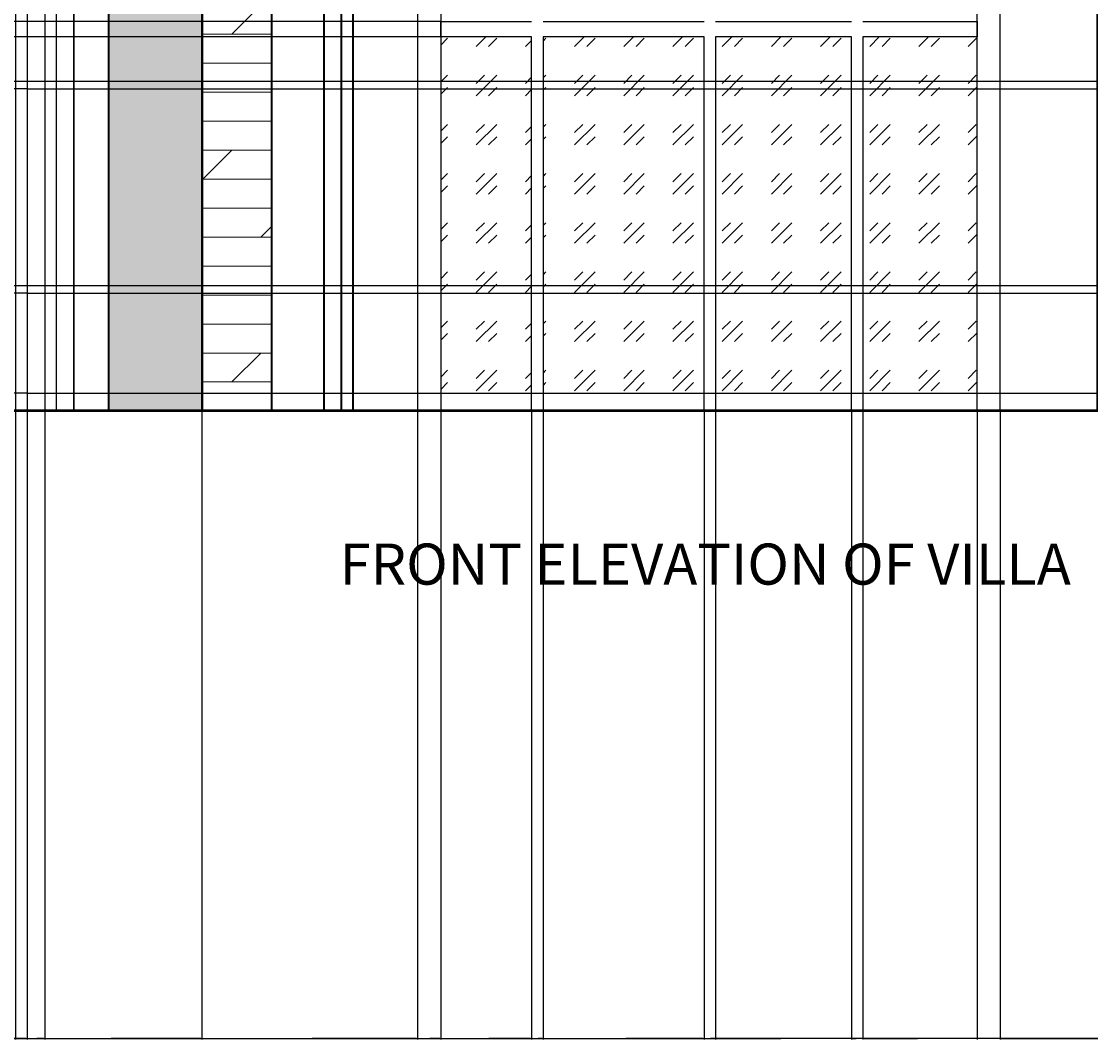
# Model space of a CAD drawing. Units: inches. Extents: x -13 to 630, y -103 to 275.
# Tile 2 of 9: x 134 to 318, y -103 to 72. Entities that reach past the tile are written whole.
import ezdxf

# ---------------------------------------------------------------- set-up
doc = ezdxf.new("R2010")
doc.units = ezdxf.units.IN
doc.header["$MEASUREMENT"] = 0
for name, color, linetype, lineweight in [('A-ANNO-DIMS', 2, 'Continuous', 18), ('A-ANNO-TEXT', 7, 'Continuous', 25), ('A-DOOR', 3, 'Continuous', 25), ('A-ELEV', 7, 'Continuous', 35), ('A-ELEV-GRND', 7, 'Continuous', 50), ('A-ELEV-PATT', 8, 'Continuous', 13), ('A-GLAZ', 4, 'Continuous', 25)]:
    doc.layers.add(name, color=color, linetype=linetype, lineweight=lineweight)
doc.styles.get("Standard").update_dxf_attribs({"font": 'arial.ttf'})
doc.dimstyles.get("Standard").update_dxf_attribs({"dimtxt": 0.18, "dimasz": 0.18, "dimexe": 0.18, "dimexo": 0.0625, "dimgap": 0.09, "dimtad": 0, "dimtih": 1, "dimtoh": 1, "dimdec": 4, "dimzin": 0, "dimdsep": 46, "dimtxsty": 'Standard', "dimcen": 0.09, "dimadec": 0, "dimazin": 0, "dimtfac": 1, "dimtdec": 4, "dimtofl": 0, "dimtmove": 0, "dimatfit": 3, "dimfxl": 1, "dimtolj": 1, "dimtzin": 0, "dimarcsym": 0})

# ---------------------------------------------------------------- blocks, each defined once
blk = doc.blocks.new('WIN-GROUND')
for points in [[(0, 0), (0, 102), (108, 102), (108, 0)], [(3, 0), (3, 99), (105, 99), (105, 0)], [(5, 0), (5, 97), (103, 97), (103, 0)], [(34.74, 56.82), (34.74, 73.49), (37, 73.49), (37, 56.82)], [(73.43, 56.82), (73.43, 73.49), (75.7, 73.49), (75.7, 56.82)], [(34.74, 55.51), (8, 55.51), (8, 56.82), (34.74, 56.82)], [(34.74, 21.58), (34.74, 55.51)], [(37, 56.82), (73.43, 56.82)], [(37, 55.51), (37, 21.58)], [(73.43, 55.51), (37, 55.51)], [(73.43, 21.58), (73.43, 55.51)], [(75.7, 56.82), (100, 56.82), (100, 55.51), (75.7, 55.51)], [(75.7, 55.51), (75.7, 21.58)], [(34.74, 20.27), (8, 20.27), (8, 21.58), (34.74, 21.58)], [(37, 21.58), (73.43, 21.58)], [(75.7, 21.58), (100, 21.58), (100, 20.27), (75.7, 20.27)], [(37, 20.27), (37, 3), (34.74, 3), (34.74, 20.27)], [(73.43, 20.27), (37, 20.27)], [(75.7, 20.27), (75.7, 3), (73.43, 3), (73.43, 20.27)]]:
    blk.add_lwpolyline(points)
for points in [[(5, 97), (103, 97), (103, 76.49), (5, 76.49)], [(5, 76.49), (103, 76.49), (103, 0), (5, 0)], [(8, 73.49), (100, 73.49), (100, 3), (8, 3)]]:
    blk.add_lwpolyline(points, close=True)
blk = doc.blocks.new('*D8')
at = {"layer": 'A-ANNO-DIMS', "color": 0, "lineweight": -2, "transparency": 16777216}
for p, q in [((142.71, 5.14), (142.71, 275.01)), ((142.89, 274.83), (153.31, 274.83)), ((164.66, 274.83), (154.24, 274.83)), ((164.84, 5.14), (164.84, 275.01))]:
    blk.add_line(p, q, dxfattribs=at)
at = {"layer": 'A-ANNO-DIMS', "color": 0, "transparency": 16777216}
for points in [[(142.89, 274.86), (142.89, 274.8), (142.71, 274.83)], [(164.66, 274.86), (164.66, 274.8), (164.84, 274.83)]]:
    blk.add_solid(points, dxfattribs=at)
at = {"layer": 'Defpoints', "color": 0, "transparency": 16777216}
for p in [(164.84, 274.83), (142.71, 5.08), (164.84, 5.08)]:
    blk.add_point(p, dxfattribs=at)
at = {"layer": 'A-ANNO-DIMS', "color": 0, "transparency": 16777216, "insert": (153.78, 274.83), "char_height": 0.18, "attachment_point": 5}
blk.add_mtext('\\A1;22.133', dxfattribs=at)
blk = doc.blocks.new('*D11')
at = {"layer": 'A-ANNO-DIMS', "color": 0, "lineweight": -2, "transparency": 16777216}
for p, q in [((16.71, 5.02), (16.71, -103.45)), ((496.71, 5.02), (496.71, -103.45)), ((16.89, -103.27), (256.42, -103.27)), ((496.53, -103.27), (257, -103.27))]:
    blk.add_line(p, q, dxfattribs=at)
at = {"layer": 'A-ANNO-DIMS', "color": 0, "transparency": 16777216}
for points in [[(16.89, -103.24), (16.89, -103.3), (16.71, -103.27)], [(496.53, -103.24), (496.53, -103.3), (496.71, -103.27)]]:
    blk.add_solid(points, dxfattribs=at)
at = {"layer": 'Defpoints', "color": 0, "transparency": 16777216}
for p in [(16.71, 5.08), (496.71, 5.08), (496.71, -103.27)]:
    blk.add_point(p, dxfattribs=at)
at = {"layer": 'A-ANNO-DIMS', "color": 0, "transparency": 16777216, "insert": (256.71, -103.27), "char_height": 0.18, "attachment_point": 5}
blk.add_mtext('\\A1;480', dxfattribs=at)
blk = doc.blocks.new('*D24')
at = {"layer": 'A-ANNO-DIMS', "color": 0, "lineweight": -2, "transparency": 16777216}
for p, q in [((164.84, 5.02), (164.84, -103.45)), ((202.02, 5.02), (202.02, -103.45)), ((165.02, -103.27), (183.04, -103.27)), ((201.84, -103.27), (183.83, -103.27))]:
    blk.add_line(p, q, dxfattribs=at)
at = {"layer": 'A-ANNO-DIMS', "color": 0, "transparency": 16777216}
for points in [[(165.02, -103.24), (165.02, -103.3), (164.84, -103.27)], [(201.84, -103.24), (201.84, -103.3), (202.02, -103.27)]]:
    blk.add_solid(points, dxfattribs=at)
at = {"layer": 'Defpoints', "color": 0, "transparency": 16777216}
for p in [(164.84, 5.08), (202.02, 5.08), (202.02, -103.27)]:
    blk.add_point(p, dxfattribs=at)
at = {"layer": 'A-ANNO-DIMS', "color": 0, "transparency": 16777216, "insert": (183.43, -103.27), "char_height": 0.18, "attachment_point": 5}
blk.add_mtext('\\A1;37.18', dxfattribs=at)
blk = doc.blocks.new('*D25')
at = {"layer": 'A-ANNO-DIMS', "color": 0, "lineweight": -2, "transparency": 16777216}
for p, q in [((202.02, 5.02), (202.02, -103.45)), ((302.53, 5.02), (302.53, -103.45)), ((202.2, -103.27), (251.89, -103.27)), ((302.35, -103.27), (252.66, -103.27))]:
    blk.add_line(p, q, dxfattribs=at)
at = {"layer": 'A-ANNO-DIMS', "color": 0, "transparency": 16777216}
for points in [[(202.2, -103.24), (202.2, -103.3), (202.02, -103.27)], [(302.35, -103.24), (302.35, -103.3), (302.53, -103.27)]]:
    blk.add_solid(points, dxfattribs=at)
at = {"layer": 'Defpoints', "color": 0, "transparency": 16777216}
for p in [(202.02, 5.08), (302.53, 5.08), (302.53, -103.27)]:
    blk.add_point(p, dxfattribs=at)
at = {"layer": 'A-ANNO-DIMS', "color": 0, "transparency": 16777216, "insert": (252.27, -103.27), "char_height": 0.18, "attachment_point": 5}
blk.add_mtext('\\A1;100.5', dxfattribs=at)
blk = doc.blocks.new('*D26')
at = {"layer": 'A-ANNO-DIMS', "color": 0, "lineweight": -2, "transparency": 16777216}
for p, q in [((302.53, 5.02), (302.53, -103.45)), ((345.31, 5.02), (345.31, -103.45)), ((302.71, -103.27), (323.52, -103.27)), ((345.13, -103.27), (324.31, -103.27))]:
    blk.add_line(p, q, dxfattribs=at)
at = {"layer": 'A-ANNO-DIMS', "color": 0, "transparency": 16777216}
for points in [[(302.71, -103.24), (302.71, -103.3), (302.53, -103.27)], [(345.13, -103.24), (345.13, -103.3), (345.31, -103.27)]]:
    blk.add_solid(points, dxfattribs=at)
at = {"layer": 'Defpoints', "color": 0, "transparency": 16777216}
for p in [(302.53, 5.08), (345.31, 5.08), (345.31, -103.27)]:
    blk.add_point(p, dxfattribs=at)
at = {"layer": 'A-ANNO-DIMS', "color": 0, "transparency": 16777216, "insert": (323.92, -103.27), "char_height": 0.18, "attachment_point": 5}
blk.add_mtext('\\A1;42.78', dxfattribs=at)
blk = doc.blocks.new('*D28')
at = {"layer": 'A-ANNO-DIMS', "color": 0, "lineweight": -2, "transparency": 16777216}
for p, q in [((302.59, 128.66), (630.03, 128.66)), ((629.85, 128.48), (629.85, 67.05)), ((629.85, 5.26), (629.85, 66.69)), ((302.59, 5.08), (630.03, 5.08))]:
    blk.add_line(p, q, dxfattribs=at)
at = {"layer": 'A-ANNO-DIMS', "color": 0, "transparency": 16777216}
for points in [[(629.82, 128.48), (629.88, 128.48), (629.85, 128.66)], [(629.82, 5.26), (629.88, 5.26), (629.85, 5.08)]]:
    blk.add_solid(points, dxfattribs=at)
at = {"layer": 'Defpoints', "color": 0, "transparency": 16777216}
for p in [(302.53, 128.66), (629.85, 128.66), (302.53, 5.08)]:
    blk.add_point(p, dxfattribs=at)
at = {"layer": 'A-ANNO-DIMS', "color": 0, "transparency": 16777216, "insert": (629.85, 66.87), "char_height": 0.18, "attachment_point": 5}
blk.add_mtext('\\A1;123.57', dxfattribs=at)
blk = doc.blocks.new('*D40')
at = {"layer": 'A-ANNO-DIMS', "color": 0, "lineweight": -2, "transparency": 16777216}
for p, q in [((205.96, 69.55), (-13.22, 69.55)), ((-13.04, 69.37), (-13.04, 37.5)), ((-13.04, 5.26), (-13.04, 37.13)), ((205.96, 5.08), (-13.22, 5.08))]:
    blk.add_line(p, q, dxfattribs=at)
at = {"layer": 'A-ANNO-DIMS', "color": 0, "transparency": 16777216}
for points in [[(-13.07, 69.37), (-13.01, 69.37), (-13.04, 69.55)], [(-13.07, 5.26), (-13.01, 5.26), (-13.04, 5.08)]]:
    blk.add_solid(points, dxfattribs=at)
at = {"layer": 'Defpoints', "color": 0, "transparency": 16777216}
for p in [(-13.04, 69.55), (206.02, 69.55), (206.02, 5.08)]:
    blk.add_point(p, dxfattribs=at)
at = {"layer": 'A-ANNO-DIMS', "color": 0, "transparency": 16777216, "insert": (-13.04, 37.31), "char_height": 0.18, "attachment_point": 5}
blk.add_mtext('\\A1;64.46', dxfattribs=at)
blk = doc.blocks.new('*D41')
at = {"layer": 'A-ANNO-DIMS', "color": 0, "lineweight": -2, "transparency": 16777216}
for p, q in [((205.96, 72.22), (-13.22, 72.22)), ((-13.04, 72.04), (-13.04, 71.07)), ((-13.04, 69.73), (-13.04, 70.7)), ((205.96, 69.55), (-13.22, 69.55))]:
    blk.add_line(p, q, dxfattribs=at)
at = {"layer": 'A-ANNO-DIMS', "color": 0, "transparency": 16777216}
for points in [[(-13.07, 72.04), (-13.01, 72.04), (-13.04, 72.22)], [(-13.07, 69.73), (-13.01, 69.73), (-13.04, 69.55)]]:
    blk.add_solid(points, dxfattribs=at)
at = {"layer": 'Defpoints', "color": 0, "transparency": 16777216}
for p in [(-13.04, 72.22), (206.02, 72.22), (206.02, 69.55)]:
    blk.add_point(p, dxfattribs=at)
at = {"layer": 'A-ANNO-DIMS', "color": 0, "transparency": 16777216, "insert": (-13.04, 70.88), "char_height": 0.18, "attachment_point": 5}
blk.add_mtext('\\A1;2.68', dxfattribs=at)
blk = doc.blocks.new('*D48')
at = {"layer": 'A-ANNO-DIMS', "color": 0, "lineweight": -2, "transparency": 16777216}
for p, q in [((202.02, 5.02), (202.02, -103.45)), ((206.02, 5.02), (206.02, -103.45)), ((202.2, -103.27), (203.87, -103.27)), ((205.84, -103.27), (204.17, -103.27))]:
    blk.add_line(p, q, dxfattribs=at)
at = {"layer": 'A-ANNO-DIMS', "color": 0, "transparency": 16777216}
for points in [[(202.2, -103.24), (202.2, -103.3), (202.02, -103.27)], [(205.84, -103.24), (205.84, -103.3), (206.02, -103.27)]]:
    blk.add_solid(points, dxfattribs=at)
at = {"layer": 'Defpoints', "color": 0, "transparency": 16777216}
for p in [(202.02, 5.08), (206.02, 5.08), (206.02, -103.27)]:
    blk.add_point(p, dxfattribs=at)
at = {"layer": 'A-ANNO-DIMS', "color": 0, "transparency": 16777216, "insert": (204.02, -103.27), "char_height": 0.18, "attachment_point": 5}
blk.add_mtext('\\A1;4', dxfattribs=at)
blk = doc.blocks.new('*D49')
at = {"layer": 'A-ANNO-DIMS', "color": 0, "lineweight": -2, "transparency": 16777216}
for p, q in [((206.02, 5.02), (206.02, -103.45)), ((221.68, 5.02), (221.68, -103.45)), ((206.2, -103.27), (213.39, -103.27)), ((221.5, -103.27), (214.3, -103.27))]:
    blk.add_line(p, q, dxfattribs=at)
at = {"layer": 'A-ANNO-DIMS', "color": 0, "transparency": 16777216}
for points in [[(206.2, -103.24), (206.2, -103.3), (206.02, -103.27)], [(221.5, -103.24), (221.5, -103.3), (221.68, -103.27)]]:
    blk.add_solid(points, dxfattribs=at)
at = {"layer": 'Defpoints', "color": 0, "transparency": 16777216}
for p in [(206.02, 5.08), (221.68, 5.08), (221.68, -103.27)]:
    blk.add_point(p, dxfattribs=at)
at = {"layer": 'A-ANNO-DIMS', "color": 0, "transparency": 16777216, "insert": (213.85, -103.27), "char_height": 0.18, "attachment_point": 5}
blk.add_mtext('\\A1;15.654', dxfattribs=at)
blk = doc.blocks.new('*D50')
at = {"layer": 'A-ANNO-DIMS', "color": 0, "lineweight": -2, "transparency": 16777216}
for p, q in [((221.68, 5.02), (221.68, -103.45)), ((223.68, 5.02), (223.68, -103.45)), ((221.86, -103.27), (222.53, -103.27)), ((223.5, -103.27), (222.82, -103.27))]:
    blk.add_line(p, q, dxfattribs=at)
at = {"layer": 'A-ANNO-DIMS', "color": 0, "transparency": 16777216}
for points in [[(221.86, -103.24), (221.86, -103.3), (221.68, -103.27)], [(223.5, -103.24), (223.5, -103.3), (223.68, -103.27)]]:
    blk.add_solid(points, dxfattribs=at)
at = {"layer": 'Defpoints', "color": 0, "transparency": 16777216}
for p in [(221.68, 5.08), (223.68, 5.08), (223.68, -103.27)]:
    blk.add_point(p, dxfattribs=at)
at = {"layer": 'A-ANNO-DIMS', "color": 0, "transparency": 16777216, "insert": (222.68, -103.27), "char_height": 0.18, "attachment_point": 5}
blk.add_mtext('\\A1;2', dxfattribs=at)
blk = doc.blocks.new('*D51')
at = {"layer": 'A-ANNO-DIMS', "color": 0, "lineweight": -2, "transparency": 16777216}
for p, q in [((223.68, 5.02), (223.68, -103.45)), ((251.44, 5.02), (251.44, -103.45)), ((223.86, -103.27), (237.16, -103.27)), ((251.26, -103.27), (237.95, -103.27))]:
    blk.add_line(p, q, dxfattribs=at)
at = {"layer": 'A-ANNO-DIMS', "color": 0, "transparency": 16777216}
for points in [[(223.86, -103.24), (223.86, -103.3), (223.68, -103.27)], [(251.26, -103.24), (251.26, -103.3), (251.44, -103.27)]]:
    blk.add_solid(points, dxfattribs=at)
at = {"layer": 'Defpoints', "color": 0, "transparency": 16777216}
for p in [(223.68, 5.08), (251.44, 5.08), (251.44, -103.27)]:
    blk.add_point(p, dxfattribs=at)
at = {"layer": 'A-ANNO-DIMS', "color": 0, "transparency": 16777216, "insert": (237.56, -103.27), "char_height": 0.18, "attachment_point": 5}
blk.add_mtext('\\A1;27.76', dxfattribs=at)
blk = doc.blocks.new('*D52')
at = {"layer": 'A-ANNO-DIMS', "color": 0, "lineweight": -2, "transparency": 16777216}
for p, q in [((251.44, 5.02), (251.44, -103.45)), ((253.44, 5.02), (253.44, -103.45)), ((251.62, -103.27), (252.29, -103.27)), ((253.26, -103.27), (252.58, -103.27))]:
    blk.add_line(p, q, dxfattribs=at)
at = {"layer": 'A-ANNO-DIMS', "color": 0, "transparency": 16777216}
for points in [[(251.62, -103.24), (251.62, -103.3), (251.44, -103.27)], [(253.26, -103.24), (253.26, -103.3), (253.44, -103.27)]]:
    blk.add_solid(points, dxfattribs=at)
at = {"layer": 'Defpoints', "color": 0, "transparency": 16777216}
for p in [(251.44, 5.08), (253.44, 5.08), (253.44, -103.27)]:
    blk.add_point(p, dxfattribs=at)
at = {"layer": 'A-ANNO-DIMS', "color": 0, "transparency": 16777216, "insert": (252.44, -103.27), "char_height": 0.18, "attachment_point": 5}
blk.add_mtext('\\A1;2', dxfattribs=at)
blk = doc.blocks.new('*D53')
at = {"layer": 'A-ANNO-DIMS', "color": 0, "lineweight": -2, "transparency": 16777216}
for p, q in [((253.44, 5.02), (253.44, -103.45)), ((276.86, 5.02), (276.86, -103.45)), ((253.62, -103.27), (264.68, -103.27)), ((276.68, -103.27), (265.61, -103.27))]:
    blk.add_line(p, q, dxfattribs=at)
at = {"layer": 'A-ANNO-DIMS', "color": 0, "transparency": 16777216}
for points in [[(253.62, -103.24), (253.62, -103.3), (253.44, -103.27)], [(276.68, -103.24), (276.68, -103.3), (276.86, -103.27)]]:
    blk.add_solid(points, dxfattribs=at)
at = {"layer": 'Defpoints', "color": 0, "transparency": 16777216}
for p in [(253.44, 5.08), (276.86, 5.08), (276.86, -103.27)]:
    blk.add_point(p, dxfattribs=at)
at = {"layer": 'A-ANNO-DIMS', "color": 0, "transparency": 16777216, "insert": (265.15, -103.27), "char_height": 0.18, "attachment_point": 5}
blk.add_mtext('\\A1;23.423', dxfattribs=at)
blk = doc.blocks.new('*D54')
at = {"layer": 'A-ANNO-DIMS', "color": 0, "lineweight": -2, "transparency": 16777216}
for p, q in [((276.86, 5.02), (276.86, -103.45)), ((278.86, 5.02), (278.86, -103.45)), ((277.04, -103.27), (277.71, -103.27)), ((278.68, -103.27), (278.01, -103.27))]:
    blk.add_line(p, q, dxfattribs=at)
at = {"layer": 'A-ANNO-DIMS', "color": 0, "transparency": 16777216}
for points in [[(277.04, -103.24), (277.04, -103.3), (276.86, -103.27)], [(278.68, -103.24), (278.68, -103.3), (278.86, -103.27)]]:
    blk.add_solid(points, dxfattribs=at)
at = {"layer": 'Defpoints', "color": 0, "transparency": 16777216}
for p in [(276.86, 5.08), (278.86, 5.08), (278.86, -103.27)]:
    blk.add_point(p, dxfattribs=at)
at = {"layer": 'A-ANNO-DIMS', "color": 0, "transparency": 16777216, "insert": (277.86, -103.27), "char_height": 0.18, "attachment_point": 5}
blk.add_mtext('\\A1;2', dxfattribs=at)
blk = doc.blocks.new('*D55')
at = {"layer": 'A-ANNO-DIMS', "color": 0, "lineweight": -2, "transparency": 16777216}
for p, q in [((278.86, 5.02), (278.86, -103.45)), ((298.53, 5.02), (298.53, -103.45)), ((279.04, -103.27), (288.24, -103.27)), ((298.35, -103.27), (289.15, -103.27))]:
    blk.add_line(p, q, dxfattribs=at)
at = {"layer": 'A-ANNO-DIMS', "color": 0, "transparency": 16777216}
for points in [[(279.04, -103.24), (279.04, -103.3), (278.86, -103.27)], [(298.35, -103.24), (298.35, -103.3), (298.53, -103.27)]]:
    blk.add_solid(points, dxfattribs=at)
at = {"layer": 'Defpoints', "color": 0, "transparency": 16777216}
for p in [(278.86, 5.08), (298.53, 5.08), (298.53, -103.27)]:
    blk.add_point(p, dxfattribs=at)
at = {"layer": 'A-ANNO-DIMS', "color": 0, "transparency": 16777216, "insert": (288.69, -103.27), "char_height": 0.18, "attachment_point": 5}
blk.add_mtext('\\A1;19.668', dxfattribs=at)
blk = doc.blocks.new('*D76')
at = {"layer": 'A-ANNO-DIMS', "color": 0, "lineweight": -2, "transparency": 16777216}
for p, q in [((110.41, 8.02), (110.41, -103.45)), ((134.71, 8.02), (134.71, -103.45)), ((110.59, -103.27), (122.24, -103.27)), ((134.53, -103.27), (122.89, -103.27))]:
    blk.add_line(p, q, dxfattribs=at)
at = {"layer": 'A-ANNO-DIMS', "color": 0, "transparency": 16777216}
for points in [[(110.59, -103.24), (110.59, -103.3), (110.41, -103.27)], [(134.53, -103.24), (134.53, -103.3), (134.71, -103.27)]]:
    blk.add_solid(points, dxfattribs=at)
at = {"layer": 'Defpoints', "color": 0, "transparency": 16777216}
for p in [(110.41, 8.08), (134.71, 8.08), (134.71, -103.27)]:
    blk.add_point(p, dxfattribs=at)
at = {"layer": 'A-ANNO-DIMS', "color": 0, "transparency": 16777216, "insert": (122.56, -103.27), "char_height": 0.18, "attachment_point": 5}
blk.add_mtext('\\A1;24.3', dxfattribs=at)
blk = doc.blocks.new('*D77')
at = {"layer": 'A-ANNO-DIMS', "color": 0, "lineweight": -2, "transparency": 16777216}
for p, q in [((134.71, 8.02), (134.71, -103.45)), ((137.71, 5.02), (137.71, -103.45)), ((134.89, -103.27), (136.06, -103.27)), ((137.53, -103.27), (136.36, -103.27))]:
    blk.add_line(p, q, dxfattribs=at)
at = {"layer": 'A-ANNO-DIMS', "color": 0, "transparency": 16777216}
for points in [[(134.89, -103.24), (134.89, -103.3), (134.71, -103.27)], [(137.53, -103.24), (137.53, -103.3), (137.71, -103.27)]]:
    blk.add_solid(points, dxfattribs=at)
at = {"layer": 'Defpoints', "color": 0, "transparency": 16777216}
for p in [(134.71, 8.08), (137.71, 5.08), (137.71, -103.27)]:
    blk.add_point(p, dxfattribs=at)
at = {"layer": 'A-ANNO-DIMS', "color": 0, "transparency": 16777216, "insert": (136.21, -103.27), "char_height": 0.18, "attachment_point": 5}
blk.add_mtext('\\A1;3', dxfattribs=at)
blk = doc.blocks.new('*D78')
at = {"layer": 'A-ANNO-DIMS', "color": 0, "lineweight": -2, "transparency": 16777216}
for p, q in [((134.77, 8.08), (630.03, 8.08)), ((629.85, 7.9), (629.85, 6.76)), ((629.85, 5.26), (629.85, 6.4)), ((137.77, 5.08), (630.03, 5.08))]:
    blk.add_line(p, q, dxfattribs=at)
at = {"layer": 'A-ANNO-DIMS', "color": 0, "transparency": 16777216}
for points in [[(629.82, 7.9), (629.88, 7.9), (629.85, 8.08)], [(629.82, 5.26), (629.88, 5.26), (629.85, 5.08)]]:
    blk.add_solid(points, dxfattribs=at)
at = {"layer": 'Defpoints', "color": 0, "transparency": 16777216}
for p in [(134.71, 8.08), (629.85, 8.08), (137.71, 5.08)]:
    blk.add_point(p, dxfattribs=at)
at = {"layer": 'A-ANNO-DIMS', "color": 0, "transparency": 16777216, "insert": (629.85, 6.58), "char_height": 0.18, "attachment_point": 5}
blk.add_mtext('\\A1;3', dxfattribs=at)
blk = doc.blocks.new('*D79')
at = {"layer": 'A-ANNO-DIMS', "color": 0, "lineweight": -2, "transparency": 16777216}
for p, q in [((134.77, 25.35), (630.03, 25.35)), ((629.85, 25.17), (629.85, 16.9)), ((629.85, 8.26), (629.85, 16.53)), ((134.77, 8.08), (630.03, 8.08))]:
    blk.add_line(p, q, dxfattribs=at)
at = {"layer": 'A-ANNO-DIMS', "color": 0, "transparency": 16777216}
for points in [[(629.82, 25.17), (629.88, 25.17), (629.85, 25.35)], [(629.82, 8.26), (629.88, 8.26), (629.85, 8.08)]]:
    blk.add_solid(points, dxfattribs=at)
at = {"layer": 'Defpoints', "color": 0, "transparency": 16777216}
for p in [(134.71, 25.35), (629.85, 25.35), (134.71, 8.08)]:
    blk.add_point(p, dxfattribs=at)
at = {"layer": 'A-ANNO-DIMS', "color": 0, "transparency": 16777216, "insert": (629.85, 16.72), "char_height": 0.18, "attachment_point": 5}
blk.add_mtext('\\A1;17.27', dxfattribs=at)
blk = doc.blocks.new('*D80')
at = {"layer": 'A-ANNO-DIMS', "color": 0, "lineweight": -2, "transparency": 16777216}
for p, q in [((134.77, 26.66), (630.03, 26.66)), ((629.85, 26.48), (629.85, 26.19)), ((629.85, 25.53), (629.85, 25.82)), ((134.77, 25.35), (630.03, 25.35))]:
    blk.add_line(p, q, dxfattribs=at)
at = {"layer": 'A-ANNO-DIMS', "color": 0, "transparency": 16777216}
for points in [[(629.82, 26.48), (629.88, 26.48), (629.85, 26.66)], [(629.82, 25.53), (629.88, 25.53), (629.85, 25.35)]]:
    blk.add_solid(points, dxfattribs=at)
at = {"layer": 'Defpoints', "color": 0, "transparency": 16777216}
for p in [(134.71, 26.66), (629.85, 26.66), (134.71, 25.35)]:
    blk.add_point(p, dxfattribs=at)
at = {"layer": 'A-ANNO-DIMS', "color": 0, "transparency": 16777216, "insert": (629.85, 26), "char_height": 0.18, "attachment_point": 5}
blk.add_mtext('\\A1;1.31', dxfattribs=at)
blk = doc.blocks.new('*D81')
at = {"layer": 'A-ANNO-DIMS', "color": 0, "lineweight": -2, "transparency": 16777216}
for p, q in [((134.77, 60.6), (630.03, 60.6)), ((629.85, 60.42), (629.85, 43.81)), ((629.85, 26.84), (629.85, 43.44)), ((134.77, 26.66), (630.03, 26.66))]:
    blk.add_line(p, q, dxfattribs=at)
at = {"layer": 'A-ANNO-DIMS', "color": 0, "transparency": 16777216}
for points in [[(629.82, 60.42), (629.88, 60.42), (629.85, 60.6)], [(629.82, 26.84), (629.88, 26.84), (629.85, 26.66)]]:
    blk.add_solid(points, dxfattribs=at)
at = {"layer": 'Defpoints', "color": 0, "transparency": 16777216}
for p in [(134.71, 60.6), (629.85, 60.6), (134.71, 26.66)]:
    blk.add_point(p, dxfattribs=at)
at = {"layer": 'A-ANNO-DIMS', "color": 0, "transparency": 16777216, "insert": (629.85, 43.63), "char_height": 0.18, "attachment_point": 5}
blk.add_mtext('\\A1;33.94', dxfattribs=at)
blk = doc.blocks.new('*D82')
at = {"layer": 'A-ANNO-DIMS', "color": 0, "lineweight": -2, "transparency": 16777216}
for p, q in [((134.77, 61.9), (630.03, 61.9)), ((629.85, 61.72), (629.85, 61.43)), ((629.85, 60.78), (629.85, 61.07)), ((134.77, 60.6), (630.03, 60.6))]:
    blk.add_line(p, q, dxfattribs=at)
at = {"layer": 'A-ANNO-DIMS', "color": 0, "transparency": 16777216}
for points in [[(629.82, 61.72), (629.88, 61.72), (629.85, 61.9)], [(629.82, 60.78), (629.88, 60.78), (629.85, 60.6)]]:
    blk.add_solid(points, dxfattribs=at)
at = {"layer": 'Defpoints', "color": 0, "transparency": 16777216}
for p in [(134.71, 61.9), (629.85, 61.9), (134.71, 60.6)]:
    blk.add_point(p, dxfattribs=at)
at = {"layer": 'A-ANNO-DIMS', "color": 0, "transparency": 16777216, "insert": (629.85, 61.25), "char_height": 0.18, "attachment_point": 5}
blk.add_mtext('\\A1;1.31', dxfattribs=at)
blk = doc.blocks.new('*D83')
at = {"layer": 'A-ANNO-DIMS', "color": 0, "lineweight": -2, "transparency": 16777216}
for p, q in [((134.77, 78.57), (630.03, 78.57)), ((629.85, 78.39), (629.85, 70.42)), ((629.85, 62.08), (629.85, 70.05)), ((134.77, 61.9), (630.03, 61.9))]:
    blk.add_line(p, q, dxfattribs=at)
at = {"layer": 'A-ANNO-DIMS', "color": 0, "transparency": 16777216}
for points in [[(629.82, 78.39), (629.88, 78.39), (629.85, 78.57)], [(629.82, 62.08), (629.88, 62.08), (629.85, 61.9)]]:
    blk.add_solid(points, dxfattribs=at)
at = {"layer": 'Defpoints', "color": 0, "transparency": 16777216}
for p in [(134.71, 78.57), (629.85, 78.57), (134.71, 61.9)]:
    blk.add_point(p, dxfattribs=at)
at = {"layer": 'A-ANNO-DIMS', "color": 0, "transparency": 16777216, "insert": (629.85, 70.24), "char_height": 0.18, "attachment_point": 5}
blk.add_mtext('\\A1;16.67', dxfattribs=at)
blk = doc.blocks.new('*D112')
at = {"layer": 'A-ANNO-DIMS', "color": 0, "lineweight": -2, "transparency": 16777216}
for p, q in [((132.66, 125.02), (132.66, -103.45)), ((164.84, 125.02), (164.84, -103.45)), ((132.84, -103.27), (148.36, -103.27)), ((164.66, -103.27), (149.15, -103.27))]:
    blk.add_line(p, q, dxfattribs=at)
at = {"layer": 'A-ANNO-DIMS', "color": 0, "transparency": 16777216}
for points in [[(132.84, -103.24), (132.84, -103.3), (132.66, -103.27)], [(164.66, -103.24), (164.66, -103.3), (164.84, -103.27)]]:
    blk.add_solid(points, dxfattribs=at)
at = {"layer": 'Defpoints', "color": 0, "transparency": 16777216}
for p in [(132.66, 125.08), (164.84, 125.08), (164.84, -103.27)]:
    blk.add_point(p, dxfattribs=at)
at = {"layer": 'A-ANNO-DIMS', "color": 0, "transparency": 16777216, "insert": (148.75, -103.27), "char_height": 0.18, "attachment_point": 5}
blk.add_mtext('\\A1;32.18', dxfattribs=at)

msp = doc.modelspace()

# ---------------------------------------------------------------- hatches: boundary and pattern name
at = {"layer": 'A-ELEV-PATT', "transparency": 33554541}
h = msp.add_hatch(dxfattribs=at)
h.set_pattern_fill('DOLMIT', color=256, scale=20)
h.paths.add_polyline_path([(345.3061, 245.0808), (164.8443, 245.0808), (164.8443, 5.0808), (176.8443, 5.0808), (176.8443, 233.0808), (333.3061, 233.0808), (333.3061, 5.0808), (345.3061, 5.0808)])
at = {"layer": 'A-ELEV-PATT'}
h = msp.add_hatch(dxfattribs=at)
h.set_pattern_fill('BRSTONE', color=256, scale=20)
h.paths.add_polyline_path([(120.6641, 172.7854), (64.9953, 172.7854, 0.41421356), (54.9953, 162.7854), (54.9953, 125.0808), (59.9953, 125.0808), (59.9953, 162.7854, -0.41421356), (64.9953, 167.7854), (120.6641, 167.7854, -0.41421356), (125.6641, 162.7854), (125.6641, 125.0808), (130.6641, 125.0808), (130.6641, 162.7854, 0.41421356)])
h.paths.add_polyline_path([(439.5513, 172.7854), (383.8825, 172.7854, 0.41421356), (373.8825, 162.7854), (373.8825, 125.0808), (378.8825, 125.0808), (378.8825, 162.7854, -0.41421356), (383.8825, 167.7854), (439.5513, 167.7854, -0.41421356), (444.5513, 162.7854), (444.5513, 125.0808), (449.5513, 125.0808), (449.5513, 162.7854, 0.41421356)])
h.paths.add_polyline_path([(364.7117, 113.0808), (484.7117, 113.0808), (484.7117, 5.0808), (496.7117, 5.0808), (496.7117, 125.0808), (345.3061, 125.0808), (345.3061, 5.0808), (364.7117, 5.0808)])
h.paths.add_polyline_path([(164.8443, 125.0808), (28.7117, 125.0808), (16.7117, 125.0808), (16.7117, 5.0808), (28.7117, 5.0808), (28.7117, 113.0808), (148.7117, 113.0808), (148.7117, 5.0808), (164.8443, 5.0808)])
h.paths.add_polyline_path([(95.1171, 223.9392), (83.8622, 223.9392), (83.8622, 206.5279), (95.1171, 206.5279)])
h.paths.add_polyline_path([(54.9212, 223.9392), (40.7186, 223.9392), (40.7186, 206.5279), (54.9212, 206.5279)])
h.paths.add_polyline_path([(463.828, 223.9392), (449.6254, 223.9392), (449.6254, 206.5279), (463.828, 206.5279)])
h.paths.add_polyline_path([(420.6843, 223.9392), (409.4295, 223.9392), (409.4295, 206.5279), (420.6843, 206.5279)])
at = {"layer": 'A-ELEV-PATT', "transparency": 33554541}
h = msp.add_hatch(dxfattribs=at)
h.set_pattern_fill('GOST_GLASS', color=256)
h.set_pattern_definition([(45, (0, 0), (8.48528, 0), [5, -7]), (45, (2.1213, 0), (8.48528, 0), [2, -10]), (45, (0, 2.1213), (8.48528, 0), [2, -10])])
h.paths.add_polyline_path([(221.6752, 69.5455), (206.0208, 69.5455), (206.0208, 5.0808), (221.6752, 5.0808)])
h.paths.add_polyline_path([(251.4352, 69.5455), (223.6752, 69.5455), (223.6752, 5.0808), (251.4352, 5.0808)])
h.paths.add_polyline_path([(276.858, 69.5455), (253.4352, 69.5455), (253.4352, 5.0808), (276.858, 5.0808)])
h.paths.add_polyline_path([(298.5258, 69.5455), (278.858, 69.5455), (278.858, 5.0808), (298.5258, 5.0808)])

# ---------------------------------------------------------------- linework, layer by layer
at = {"layer": 'A-DOOR'}
for points in [[(221.6752, 5.0808), (221.6752, 69.5455)], [(223.6752, 69.5455), (223.6752, 5.0808)], [(251.4352, 69.5455), (223.6752, 69.5455)], [(251.4352, 5.0808), (251.4352, 69.5455)], [(253.4352, 69.5455), (253.4352, 5.0808)], [(276.858, 69.5455), (253.4352, 69.5455)], [(278.858, 69.5455), (278.858, 5.0808), (276.858, 5.0808), (276.858, 69.5455)]]:
    msp.add_lwpolyline(points, dxfattribs=at)
at = {"layer": 'A-ELEV'}
msp.add_line((164.8443, 5.0808), (345.3061, 5.0808), dxfattribs=at)
for points in [[(345.3061, 5.0808), (345.3061, 245.0808), (164.8443, 245.0808), (164.8443, 5.0808)], [(333.3061, 5.0808), (333.3061, 233.0808), (176.8443, 233.0808), (176.8443, 5.0808)], [(324.3061, 5.0808), (324.3061, 224.0808), (185.8443, 224.0808), (185.8443, 5.0808)], [(321.3061, 5.0808), (321.3061, 221.0808), (188.8443, 221.0808), (188.8443, 5.0808)], [(319.3061, 5.0808), (319.3061, 219.0808), (190.8443, 219.0808), (190.8443, 5.0808)], [(28.7117, 5.0808), (28.7117, 113.0808), (148.7117, 113.0808), (148.7117, 5.0808)]]:
    msp.add_lwpolyline(points, dxfattribs=at)
at = {"layer": 'A-ELEV-GRND'}
msp.add_line((16.7117, 5.0808), (496.7117, 5.0808), dxfattribs=at)
at = {"layer": 'A-GLAZ'}
for p, q in [((202.0208, 203.9359), (202.0208, 5.0808)), ((302.5258, 5.0808), (302.5258, 203.9359)), ((206.0208, 128.6551), (206.0208, 5.0808)), ((298.5258, 5.0808), (298.5258, 128.6551)), ((202.0208, 5.0808), (302.5258, 5.0808))]:
    msp.add_line(p, q, dxfattribs=at)
for points in [[(221.6752, 69.5455), (206.0208, 69.5455), (206.0208, 72.223), (221.6752, 72.223)], [(223.6752, 72.223), (251.4352, 72.223)], [(253.4352, 72.223), (276.858, 72.223)], [(278.858, 72.223), (298.5258, 72.223), (298.5258, 69.5455), (278.858, 69.5455)]]:
    msp.add_lwpolyline(points, dxfattribs=at)

# ---------------------------------------------------------------- block references
msp.add_blockref('WIN-GROUND', (34.712, 5.081), dxfattribs=at)

# ---------------------------------------------------------------- texts
at = {"layer": 'A-ANNO-TEXT'}
msp.add_text('FRONT ELEVATION OF VILLA', height=7.09027, dxfattribs=at).set_placement((188.58, -24.9622))

# ---------------------------------------------------------------- dimensions: what is measured, and where the dimension line sits
at = {"layer": 'A-ANNO-DIMS'}
for base, p1, p2, override, picture, middle in [((164.8443, 274.8308), (142.7117, 5.0808), (164.8443, 5.0808), {"dimdec": 3, "dimlfac": 1, "dimrnd": 0, "dimzin": 0, "dimdsep": 46, "dimlunit": 2}, '*D8', (153.778, 274.8308)), ((164.8443, -103.2746), (132.6641, 125.0808), (164.8443, 125.0808), {"dimdec": 2, "dimlfac": 1, "dimrnd": 0, "dimzin": 0, "dimdsep": 46, "dimlunit": 2}, '*D112', (148.7542, -103.2746)), ((134.7117, -103.2746), (110.4122, 8.0808), (134.7117, 8.0808), {"dimdec": 1, "dimlfac": 1, "dimrnd": 0, "dimzin": 0, "dimdsep": 46, "dimlunit": 2}, '*D76', (122.562, -103.2746)), ((137.7117, -103.2746), (134.7117, 8.0808), (137.7117, 5.0808), {"dimdec": 0, "dimlfac": 1, "dimrnd": 0, "dimzin": 0, "dimdsep": 46, "dimlunit": 2}, '*D77', (136.2117, -103.2746)), ((496.7117, -103.2746), (16.7117, 5.0808), (496.7117, 5.0808), {"dimdec": 0, "dimlfac": 1, "dimrnd": 0, "dimzin": 0, "dimdsep": 46, "dimlunit": 2}, '*D11', (256.7117, -103.2746)), ((202.0208, -103.2746), (164.8443, 5.0808), (202.0208, 5.0808), {"dimdec": 2, "dimlfac": 1, "dimrnd": 0, "dimzin": 0, "dimdsep": 46, "dimlunit": 2}, '*D24', (183.4325, -103.2746)), ((302.5258, -103.2746), (202.0208, 5.0808), (302.5258, 5.0808), {"dimdec": 1, "dimlfac": 1, "dimrnd": 0, "dimzin": 0, "dimdsep": 46, "dimlunit": 2}, '*D25', (252.2733, -103.2746)), ((206.0208, -103.2746), (202.0208, 5.0808), (206.0208, 5.0808), {"dimdec": 0, "dimlfac": 1, "dimrnd": 0, "dimzin": 0, "dimdsep": 46, "dimlunit": 2}, '*D48', (204.0208, -103.2746)), ((221.6752, -103.2746), (206.0208, 5.0808), (221.6752, 5.0808), {"dimdec": 3, "dimlfac": 1, "dimrnd": 0, "dimzin": 0, "dimdsep": 46, "dimlunit": 2}, '*D49', (213.848, -103.2746)), ((223.6752, -103.2746), (221.6752, 5.0808), (223.6752, 5.0808), {"dimdec": 0, "dimlfac": 1, "dimrnd": 0, "dimzin": 0, "dimdsep": 46, "dimlunit": 2}, '*D50', (222.6752, -103.2746)), ((251.4352, -103.2746), (223.6752, 5.0808), (251.4352, 5.0808), {"dimdec": 2, "dimlfac": 1, "dimrnd": 0, "dimzin": 0, "dimdsep": 46, "dimlunit": 2}, '*D51', (237.5552, -103.2746)), ((253.4352, -103.2746), (251.4352, 5.0808), (253.4352, 5.0808), {"dimdec": 0, "dimlfac": 1, "dimrnd": 0, "dimzin": 0, "dimdsep": 46, "dimlunit": 2}, '*D52', (252.4352, -103.2746)), ((276.858, -103.2746), (253.4352, 5.0808), (276.858, 5.0808), {"dimdec": 3, "dimlfac": 1, "dimrnd": 0, "dimzin": 0, "dimdsep": 46, "dimlunit": 2}, '*D53', (265.1466, -103.2746)), ((278.858, -103.2746), (276.858, 5.0808), (278.858, 5.0808), {"dimdec": 0, "dimlfac": 1, "dimrnd": 0, "dimzin": 0, "dimdsep": 46, "dimlunit": 2}, '*D54', (277.858, -103.2746)), ((298.5258, -103.2746), (278.858, 5.0808), (298.5258, 5.0808), {"dimdec": 3, "dimlfac": 1, "dimrnd": 0, "dimzin": 0, "dimdsep": 46, "dimlunit": 2}, '*D55', (288.6919, -103.2746)), ((345.3061, -103.2746), (302.5258, 5.0808), (345.3061, 5.0808), {"dimdec": 2, "dimlfac": 1, "dimrnd": 0, "dimzin": 0, "dimdsep": 46, "dimlunit": 2}, '*D26', (323.9159, -103.2746))]:
    dim = msp.add_linear_dim(base=base, p1=p1, p2=p2, dimstyle='Standard', override=override, dxfattribs=at)
    dim.commit()
    dim.dimension.update_dxf_attribs({"geometry": picture, "text_midpoint": middle})
for base, p1, p2, override, picture, middle in [((629.8508, 128.6551), (302.5258, 5.0808), (302.5258, 128.6551), {"dimdec": 2, "dimlfac": 1, "dimrnd": 0, "dimzin": 0, "dimdsep": 46, "dimlunit": 2}, '*D28', (629.8508, 66.868)), ((629.8508, 78.5713), (134.7117, 61.902), (134.7117, 78.5713), {"dimdec": 2, "dimlfac": 1, "dimrnd": 0, "dimzin": 0, "dimdsep": 46, "dimlunit": 2}, '*D83', (629.8508, 70.2366)), ((-13.0383, 72.223), (206.0208, 69.5455), (206.0208, 72.223), {"dimdec": 2, "dimlfac": 1, "dimrnd": 0, "dimzin": 0, "dimdsep": 46, "dimlunit": 2}, '*D41', (-13.0383, 70.8842)), ((-13.0383, 69.5455), (206.0208, 5.0808), (206.0208, 69.5455), {"dimdec": 2, "dimlfac": 1, "dimrnd": 0, "dimzin": 0, "dimdsep": 46, "dimlunit": 2}, '*D40', (-13.0383, 37.3131)), ((629.8508, 61.902), (134.7117, 60.5952), (134.7117, 61.902), {"dimdec": 2, "dimlfac": 1, "dimrnd": 0, "dimzin": 0, "dimdsep": 46, "dimlunit": 2}, '*D82', (629.8508, 61.2486)), ((629.8508, 60.5952), (134.7117, 26.6567), (134.7117, 60.5952), {"dimdec": 2, "dimlfac": 1, "dimrnd": 0, "dimzin": 0, "dimdsep": 46, "dimlunit": 2}, '*D81', (629.8508, 43.6259)), ((629.8508, 26.6567), (134.7117, 25.3499), (134.7117, 26.6567), {"dimdec": 2, "dimlfac": 1, "dimrnd": 0, "dimzin": 0, "dimdsep": 46, "dimlunit": 2}, '*D80', (629.8508, 26.0033)), ((629.8508, 25.3499), (134.7117, 8.0808), (134.7117, 25.3499), {"dimdec": 2, "dimlfac": 1, "dimrnd": 0, "dimzin": 0, "dimdsep": 46, "dimlunit": 2}, '*D79', (629.8508, 16.7154)), ((629.8508, 8.0808), (137.7117, 5.0808), (134.7117, 8.0808), {"dimdec": 0, "dimlfac": 1, "dimrnd": 0, "dimzin": 0, "dimdsep": 46, "dimlunit": 2}, '*D78', (629.8508, 6.5808))]:
    dim = msp.add_linear_dim(base=base, p1=p1, p2=p2, angle=90, dimstyle='Standard', override=override, dxfattribs=at)
    dim.commit()
    dim.dimension.update_dxf_attribs({"geometry": picture, "text_midpoint": middle})

doc.saveas('drawing.dxf')
